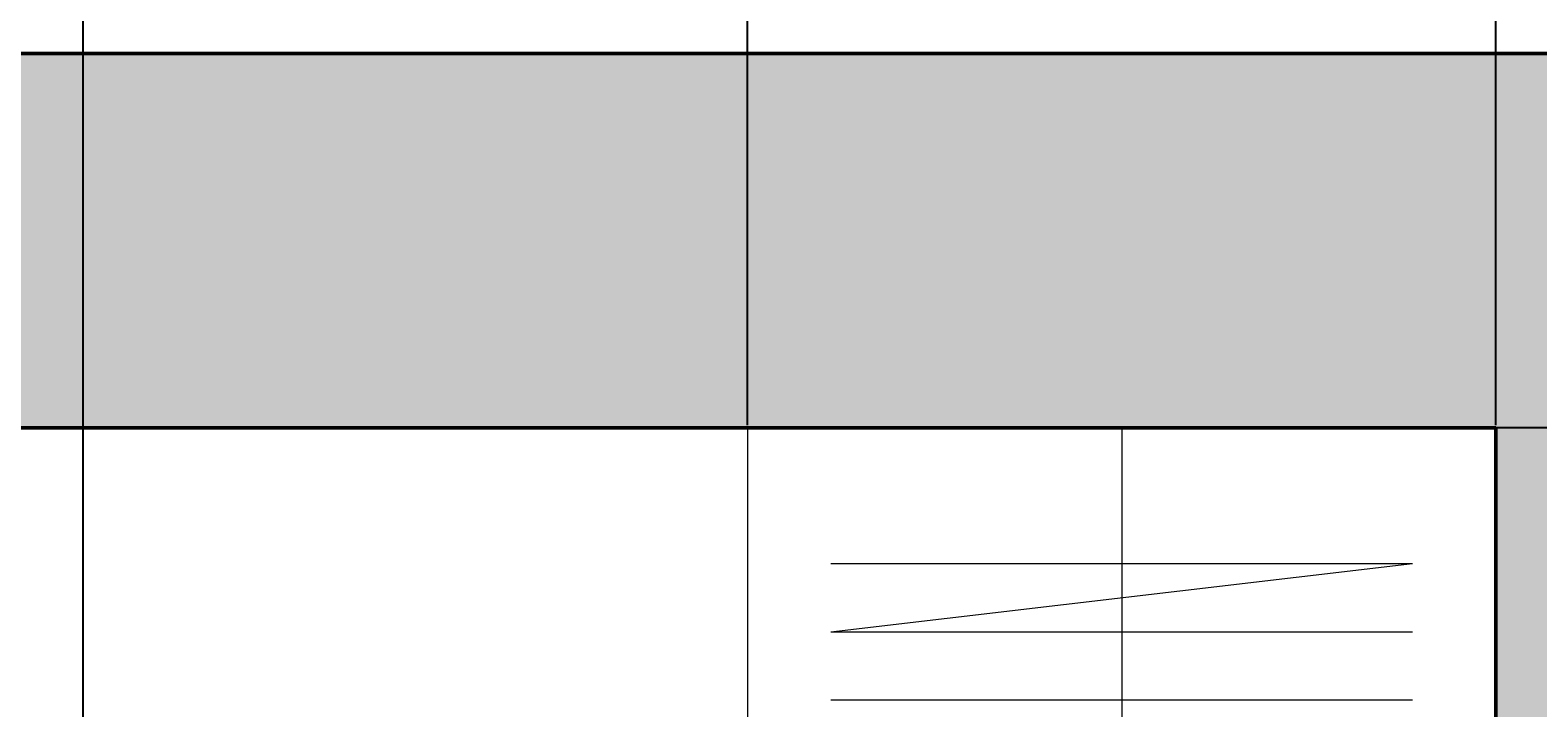
# Model space of a CAD drawing. Units: inches. Extents: x 2307 to 2544, y 2171 to 2540.
# Tile 28 of 52: x 2416 to 2453, y 2505 to 2521. Entities that reach past the tile are written whole.
import ezdxf

# ---------------------------------------------------------------- set-up
doc = ezdxf.new("R2010")
doc.units = ezdxf.units.IN
for name, color, linetype, lineweight in [('A-ANNO-DIMS', 2, 'Continuous', 18), ('A-FLOR-CASE', 9, 'Continuous', 18), ('A-WALL', 7, 'Continuous', 50)]:
    doc.layers.add(name, color=color, linetype=linetype, lineweight=lineweight)
doc.layers.add('A-WALL-PATT', color=18, linetype='Continuous', lineweight=13, true_color=0x000000)
doc.styles.get("Standard").update_dxf_attribs({"font": 'arial.ttf'})
doc.dimstyles.get("Standard").update_dxf_attribs({"dimtxt": 0.18, "dimasz": 0.18, "dimexe": 0.18, "dimexo": 0.0625, "dimgap": 0.09, "dimtad": 0, "dimtih": 1, "dimtoh": 1, "dimdec": 4, "dimzin": 0, "dimdsep": 46, "dimtxsty": 'Standard', "dimcen": 0.09, "dimadec": 0, "dimazin": 0, "dimtfac": 1, "dimtdec": 4, "dimtofl": 0, "dimtmove": 0, "dimatfit": 3, "dimfxl": 1, "dimtolj": 1, "dimtzin": 0, "dimarcsym": 0})

# ---------------------------------------------------------------- blocks, each defined once
blk = doc.blocks.new('WARDROBE-72X18IN')
for p, q in [((0, 72), (0, 0)), ((18, 72), (0, 72)), ((9, 72), (9, 0)), ((18, 0), (18, 72)), ((16, 68.727), (2, 68.727)), ((16, 68.727), (2, 67.09)), ((16, 67.09), (2, 67.09)), ((16, 65.454), (2, 65.454))]:
    blk.add_line(p, q)
blk = doc.blocks.new('*D45')
at = {"layer": 'A-ANNO-DIMS', "color": 0, "lineweight": -2, "transparency": 16777216}
for p, q in [((2335.696, 2511.572), (2335.696, 2530.84)), ((2451.696, 2511.572), (2451.696, 2530.84)), ((2335.876, 2530.66), (2393.416, 2530.66)), ((2451.516, 2530.66), (2393.976, 2530.66))]:
    blk.add_line(p, q, dxfattribs=at)
at = {"layer": 'A-ANNO-DIMS', "color": 0, "transparency": 16777216}
for points in [[(2335.876, 2530.69), (2335.876, 2530.63), (2335.696, 2530.66)], [(2451.516, 2530.69), (2451.516, 2530.63), (2451.696, 2530.66)]]:
    blk.add_solid(points, dxfattribs=at)
at = {"layer": 'Defpoints', "color": 0, "transparency": 16777216}
for p in [(2451.696, 2530.66), (2335.696, 2511.51), (2451.696, 2511.51)]:
    blk.add_point(p, dxfattribs=at)
at = {"layer": 'A-ANNO-DIMS', "color": 0, "transparency": 16777216, "insert": (2393.696, 2530.66), "char_height": 0.18, "attachment_point": 5}
blk.add_mtext('\\A1;116', dxfattribs=at)
blk = doc.blocks.new('*D48')
at = {"layer": 'A-ANNO-DIMS', "color": 0, "lineweight": -2, "transparency": 16777216}
for p, q in [((2455.633, 2511.51), (2307.366, 2511.51)), ((2307.546, 2511.33), (2307.546, 2475.69)), ((2307.546, 2439.69), (2307.546, 2475.329)), ((2455.633, 2439.51), (2307.366, 2439.51))]:
    blk.add_line(p, q, dxfattribs=at)
at = {"layer": 'A-ANNO-DIMS', "color": 0, "transparency": 16777216}
for points in [[(2307.516, 2511.33), (2307.576, 2511.33), (2307.546, 2511.51)], [(2307.516, 2439.69), (2307.576, 2439.69), (2307.546, 2439.51)]]:
    blk.add_solid(points, dxfattribs=at)
at = {"layer": 'Defpoints', "color": 0, "transparency": 16777216}
for p in [(2307.546, 2511.51), (2455.696, 2511.51), (2455.696, 2439.51)]:
    blk.add_point(p, dxfattribs=at)
at = {"layer": 'A-ANNO-DIMS', "color": 0, "transparency": 16777216, "insert": (2307.546, 2475.51), "char_height": 0.18, "attachment_point": 5}
blk.add_mtext('\\A1;72', dxfattribs=at)
blk = doc.blocks.new('*D69')
at = {"layer": 'A-ANNO-DIMS', "color": 0, "lineweight": -2, "transparency": 16777216}
for p, q in [((2417.708, 2490.237), (2417.708, 2540.345)), ((2417.888, 2540.165), (2425.247, 2540.165)), ((2433.516, 2540.165), (2426.157, 2540.165)), ((2433.696, 2511.572), (2433.696, 2540.345))]:
    blk.add_line(p, q, dxfattribs=at)
at = {"layer": 'A-ANNO-DIMS', "color": 0, "transparency": 16777216}
for points in [[(2417.888, 2540.195), (2417.888, 2540.135), (2417.708, 2540.165)], [(2433.516, 2540.195), (2433.516, 2540.135), (2433.696, 2540.165)]]:
    blk.add_solid(points, dxfattribs=at)
at = {"layer": 'Defpoints', "color": 0, "transparency": 16777216}
for p in [(2433.696, 2540.165), (2433.696, 2511.51), (2417.708, 2490.174)]:
    blk.add_point(p, dxfattribs=at)
at = {"layer": 'A-ANNO-DIMS', "color": 0, "transparency": 16777216, "insert": (2425.702, 2540.165), "char_height": 0.18, "attachment_point": 5}
blk.add_mtext('\\A1;15.987', dxfattribs=at)

msp = doc.modelspace()

# ---------------------------------------------------------------- hatches: boundary and pattern name
at = {"layer": 'A-WALL-PATT'}
h = msp.add_hatch(color=256, dxfattribs=at)
h.dxf.hatch_style = 1
h.paths.add_polyline_path([(2433.6935, 2199.5096), (2415.6423, 2199.5096), (2415.6423, 2190.5096), (2433.7832, 2190.5096)], flags=17)
h.paths.add_polyline_path([(2367.6423, 2199.5096), (2335.6958, 2199.5096), (2335.6958, 2307.3983), (2326.6958, 2307.3983), (2326.6958, 2190.5096), (2367.6423, 2190.5096)])
h.paths.add_polyline_path([(2524.6958, 2520.5096), (2496.7832, 2520.5096), (2496.7832, 2515.5149), (2472.7832, 2515.5149), (2472.7832, 2520.5096), (2415.4028, 2520.5096), (2415.4028, 2511.5096), (2451.6958, 2511.5096), (2451.6958, 2439.5096), (2451.6958, 2391.5096), (2445.6958, 2391.5096), (2445.6958, 2387.5096), (2455.6958, 2387.5096), (2455.6958, 2435.5096), (2461.6958, 2435.5096), (2461.6958, 2439.5096), (2455.6958, 2439.5096), (2455.6958, 2511.5096), (2515.6958, 2511.5096), (2515.6958, 2439.5096), (2491.6958, 2439.5096), (2491.6958, 2435.5096), (2515.6958, 2435.5096), (2515.6958, 2319.5096), (2451.6958, 2319.5096), (2451.6958, 2281.5096), (2481.6958, 2281.5096), (2481.6958, 2225.5096), (2485.6958, 2225.5096), (2485.6958, 2285.5096), (2455.6958, 2285.5096), (2455.6958, 2315.5096), (2515.6958, 2315.5096), (2515.6958, 2199.5096), (2469.6952, 2199.5096), (2469.785, 2190.5096), (2524.6958, 2190.5096)])

# ---------------------------------------------------------------- linework, layer by layer
at = {"layer": 'A-WALL'}
for p in [(2335.6958, 2511.5096), (2451.6958, 2391.5096)]:
    msp.add_line(p, (2451.6958, 2511.5096), dxfattribs=at)
msp.add_lwpolyline([(2433.7832, 2190.5096), (2326.6958, 2190.5096), (2326.6958, 2520.5096), (2524.6958, 2520.5096), (2524.6958, 2190.5096), (2469.785, 2190.5096)], dxfattribs=at)

# ---------------------------------------------------------------- block references
at = {"layer": 'A-FLOR-CASE'}
msp.add_blockref('WARDROBE-72X18IN', (2433.696, 2439.51), dxfattribs=at)

# ---------------------------------------------------------------- dimensions: what is measured, and where the dimension line sits
at = {"layer": 'A-ANNO-DIMS'}
for base, p1, p2, override, picture, middle in [((2433.6958, 2540.1649), (2417.7084, 2490.1742), (2433.6958, 2511.5096), {"dimdec": 3, "dimlfac": 1, "dimrnd": 0, "dimzin": 0, "dimdsep": 46, "dimlunit": 2}, '*D69', (2425.7021, 2540.1649)), ((2451.6958, 2530.6596), (2335.6958, 2511.5096), (2451.6958, 2511.5096), {"dimdec": 0, "dimlfac": 1, "dimrnd": 0, "dimzin": 0, "dimdsep": 46, "dimlunit": 2}, '*D45', (2393.6958, 2530.6596))]:
    dim = msp.add_linear_dim(base=base, p1=p1, p2=p2, dimstyle='Standard', override=override, dxfattribs=at)
    dim.commit()
    dim.dimension.update_dxf_attribs({"geometry": picture, "text_midpoint": middle})
dim = msp.add_linear_dim(base=(2307.5458, 2511.5096), p1=(2455.6958, 2439.5096), p2=(2455.6958, 2511.5096), angle=90, dimstyle='Standard', override={"dimdec": 0, "dimlfac": 1, "dimrnd": 0, "dimzin": 0, "dimdsep": 46, "dimlunit": 2}, dxfattribs=at)
dim.commit()
dim.dimension.update_dxf_attribs({"geometry": '*D48', "text_midpoint": (2307.5458, 2475.5096)})

doc.saveas('drawing.dxf')
